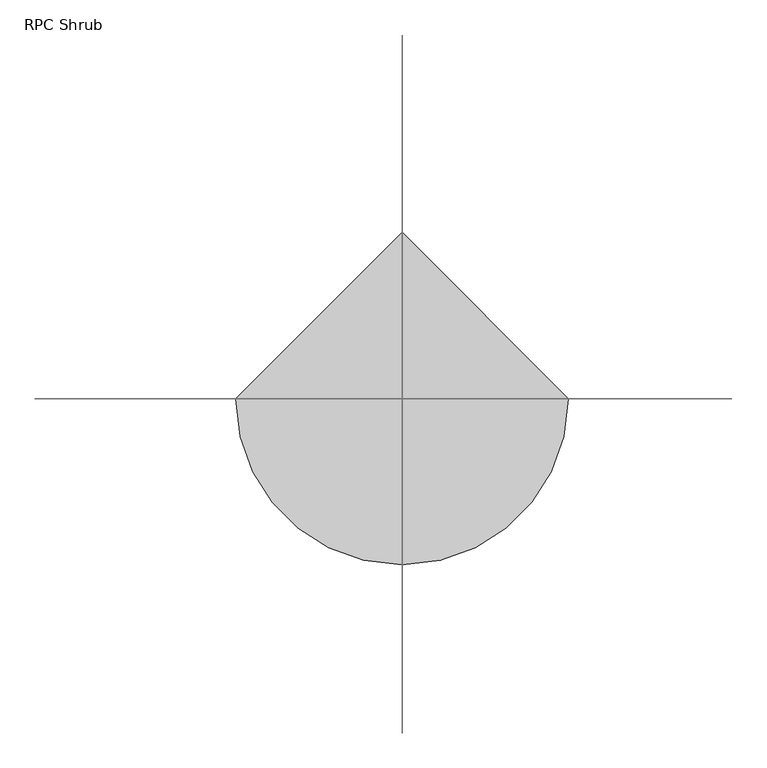
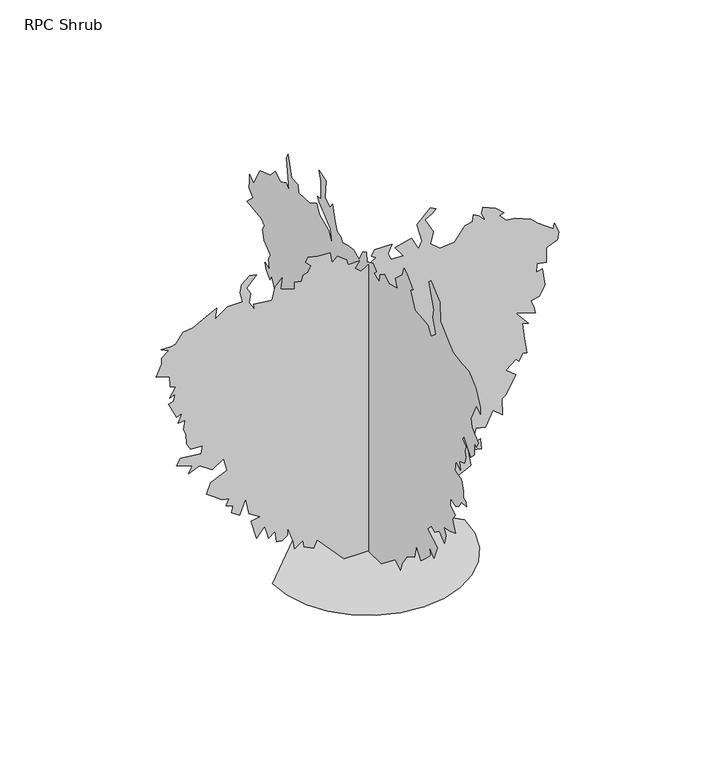
"""IFC4 building model written with IfcOpenShell, lengths in millimetres: geographic element geometry, RPC Shrub."""

from ifc_helpers import new_model, si_unit, origin, place, context, project, spatial, triangles, source, transform, mapped, element, save


def rpc_shrub_9ef344a8(model_context):
    return source(origin(), model_context, "Body", "Tessellation", [
        triangles([(-63.9369313, 2.6e-06, 2.5813025), (-98.6351404, 1.9e-06, 41.3616468), (-133.3335948, 1.1e-06, 80.1421467), (-143.538813, 2.7e-06, 59.7314513), (-168.0315495, 3.1e-06, 71.9778149), (-170.0726858, 2.1e-06, 90.347365), (-192.5245312, 3.9e-06, 76.0598514), (-194.5656857, 2.9e-06, 94.4296558), (-210.8940858, 9e-07, 139.3333375), (-210.8940858, 2.1e-06, 118.9223832), (-225.1818402, 3.4e-06, 108.7171649), (-239.469104, 3.9e-06, 110.7583103), (-243.5513948, 2.2e-06, 141.3742286), (-260.2917792, 3.7e-06, 128.4682213), (-264.2033864, 3e-06, 143.1357217), (-270.0860397, 2e-06, 163.8260649), (-290.4949502, 4.4e-06, 139.3333375), (-304.7824684, 2e-06, 190.3599468), (-282.331386, 8e-07, 194.4422376), (-310.9064223, 9e-07, 212.8117922), (-319.0699865, -1.4e-06, 257.7162279), (-335.3996584, 1.7e-06, 216.894083), (-355.8110942, 1.8e-06, 231.181583), (-351.7293303, 5e-07, 249.5511376), (-370.0986305, 9e-07, 255.674056), (-361.9325229, -4e-07, 272.003746), (-380.3043303, 2e-07, 276.0855281), (-401.9400736, 2e-07, 291.703997), (-421.1247311, 3e-07, 304.6605463), (-410.918995, -1.9e-06, 333.2355826), (-368.1987102, -4.9e-06, 351.9401459), (-376.2200229, -6.6e-06, 386.3038187), (-406.8371947, -4.1e-06, 367.9345184), (-439.493995, -4.1e-06, 390.385619), (-468.0690313, -2.1e-06, 378.137711), (-457.8632953, -3.5e-06, 394.4673829), (-498.6862032, -2.7e-06, 410.7970548), (-488.4805035, -4.1e-06, 427.1242195), (-435.4122311, -6.1e-06, 421.0002474), (-431.3304308, -7.5e-06, 441.4117195), (-461.9450955, -6.2e-06, 443.4538914), (-472.1508316, -6.9e-06, 461.8231553), (-474.1929671, -8.4e-06, 488.3560198), (-480.3169393, -9e-06, 502.6435561), (-476.2325955, -1.06e-05, 527.1367922), (-495.4832737, -9.7e-06, 526.35192), (-484.3987032, -1.16e-05, 549.5878564), (-498.6862032, -1.06e-05, 543.466464), (-519.0951319, -1.23e-05, 586.3290004), (-506.8497674, -1.3e-05, 590.4107643), (-502.7680035, -1.43e-05, 608.7800646), (-517.0555035, -1.33e-05, 602.6561288), (-500.7258316, -1.55e-05, 627.1493649), (-516.1995237, -1.52e-05, 634.2689884), (-517.0555035, -1.68e-05, 661.848337), (-551.7544756, -1.59e-05, 672.0540367), (-537.4644321, -1.84e-05, 702.6687378), (-538.1857907, -1.94e-05, 720.3319038), (-519.0951319, -2.1e-05, 733.2859097), (-539.506604, -2.07e-05, 743.4916094), (-512.7375257, -2.18e-05, 742.0895147), (-500.7258316, -2.25e-05, 745.5312378), (-482.3565313, -2.49e-05, 772.0666094), (-455.8236669, -2.62e-05, 774.1062378), (-423.1668666, -2.87e-05, 792.4755381), (-395.1176339, -3.08e-05, 806.3871162), (-398.6736305, -2.9e-05, 778.1880381), (-366.0168303, -3.17e-05, 800.6416821), (-327.2360942, -3.34e-05, 800.6416821), (-334.4166515, -3.47e-05, 827.9339842), (-330.1088113, -3.62e-05, 849.0616917), (-308.8667939, -3.81e-05, 865.9552826), (-290.4949502, -3.87e-05, 861.8734823), (-317.5358142, -3.58e-05, 834.0731443), (-306.8246221, -3.53e-05, 816.9688105), (-310.9064223, -3.36e-05, 792.4755381), (-296.6189042, -3.29e-05, 770.0245102), (-298.6610579, -3.37e-05, 784.3120102), (-251.0357672, -3.54e-05, 778.383593), (-243.5513948, -3.77e-05, 810.8473818), (-225.1818402, -3.97e-05, 831.2563105), (-228.2958943, -3.78e-05, 801.312208), (-192.5245312, -3.86e-05, 788.3937378), (-192.5245312, -3.97e-05, 806.7630381), (-173.5245645, -4.03e-05, 803.1613684), (-170.0726858, -4.14e-05, 819.0109823), (-157.8260678, -4.22e-05, 823.0927099), (-149.662004, -4.34e-05, 837.3802826), (-163.9495131, -4.36e-05, 851.6677826), (-157.8260678, -4.46e-05, 863.9131107), (-131.292195, -4.54e-05, 857.7916821), (-100.6760314, -4.66e-05, 855.7495102), (-94.5528496, -4.52e-05, 827.1745102), (-80.2653314, -4.65e-05, 839.4223818), (-56.9158573, -4.65e-05, 821.1673914), (-53.7314587, -4.57e-05, 806.7630381), (-23.1153655, -4.71e-05, 806.7630381), (-35.3616542, -4.56e-05, 790.4359097), (-19.0331746, -4.54e-05, 776.1484097), (19.7470164, -4.86e-05, 800.6416821), (7.5007532, -4.85e-05, 808.8052099), (15.1231208, -4.98e-05, 823.890263), (60.5683824, -5.17e-05, 823.0927099), (50.5958261, -4.99e-05, 799.816151), (58.5274868, -4.92e-05, 782.2723818), (91.1845505, -5.05e-05, 780.2302099), (68.732964, -5.13e-05, 810.8473818), (111.5952414, -5.38e-05, 821.0506107), (129.9650504, -5.25e-05, 786.3541821), (138.9452253, -5.4e-05, 804.6625122), (125.8830048, -5.64e-05, 853.7099545), (160.581223, -6e-05, 888.4063831), (174.868723, -6.01e-05, 880.2427826), (164.6635138, -5.91e-05, 870.0370829), (146.2937048, -5.76e-05, 859.8313105), (168.7455503, -5.62e-05, 819.0109823), (161.0930195, -5.4e-05, 788.6985884), (185.0742047, -5.39e-05, 767.9848818), (203.4434868, -5.48e-05, 770.0245102), (223.8544503, -5.58e-05, 772.0666094), (250.3885683, -5.9e-05, 806.7630381), (269.7101179, -6.01e-05, 811.2766434), (272.8393963, -6.13e-05, 829.2166821), (285.0872861, -6.15e-05, 823.0927099), (304.0839645, -6.12e-05, 803.1613684), (293.2508503, -6.21e-05, 827.1745102), (297.3326324, -6.31e-05, 841.4620102), (329.9894508, -6.37e-05, 827.1745102), (351.394031, -6.35e-05, 807.9441433), (340.0529354, -6.27e-05, 803.4457987), (358.5644508, -6.24e-05, 784.3120102), (381.0180948, -6.33e-05, 782.2723818), (422.1051581, -6.41e-05, 765.7470823), (440.2077596, -6.38e-05, 747.5734097), (481.0306675, -6.39e-05, 718.9984097), (483.0702959, -6.48e-05, 733.2859097), (495.3181675, -6.36e-05, 704.710837), (491.2364036, -6.23e-05, 684.2994375), (462.6588238, -6.03e-05, 672.0540367), (462.6588238, -5.8e-05, 633.273337), (438.1681312, -5.71e-05, 637.3550646), (436.1259593, -5.57e-05, 614.9040367), (452.4556312, -5.67e-05, 618.9857643), (458.5770598, -5.41e-05, 572.041464), (444.2895235, -5.19e-05, 545.5060925), (421.8384593, -5.07e-05, 541.4242922), (430.0020235, -4.98e-05, 521.0128201), (434.0863309, -4.91e-05, 504.6856916), (383.0577232, -4.78e-05, 521.0128201), (415.7145235, -4.69e-05, 482.2346274), (399.3873951, -4.64e-05, 486.3163914), (405.5087874, -4.42e-05, 443.4538914), (411.6327232, -4.2e-05, 402.6309471), (401.4269872, -4.17e-05, 404.673119), (391.2212874, -4.01e-05, 386.3038187), (383.0577232, -4.03e-05, 394.4673829), (356.5248588, -3.79e-05, 374.0559471), (383.0577232, -3.77e-05, 351.6048466), (356.5248588, -3.39e-05, 306.7001747), (346.3191227, -3.29e-05, 298.5365923), (348.3587511, -3.03e-05, 253.6334284), (323.4463909, -3.05e-05, 274.9933165), (303.4565864, -2.73e-05, 235.2636194), (278.9633503, -2.66e-05, 241.3868104), (266.8272088, -2.35e-05, 199.2829668), (291.2086966, -2.52e-05, 208.7297557), (293.2508503, -2.36e-05, 180.1547194), (258.5518782, -2.25e-05, 188.3190466), (266.7179858, -2.02e-05, 143.415374), (232.0187775, -1.77e-05, 127.0867195), (215.6903774, -1.54e-05, 100.5528377), (197.3205684, -1.5e-05, 106.6760195), (191.1973775, -1.2e-05, 61.7723423), (176.9098775, -1.3e-05, 88.306474), (150.3759956, -8.8e-06, 37.2796104), (132.0059414, -8.8e-06, 51.5671195), (68.732964, -3.2e-06, 2.5813025), (5e-07, 58.5086925, 0.0), (5.6e-06, 119.7410287, 55.1089), (6.1e-06, 137.5863239, 49.658565), (5.6e-06, 170.7679014, 104.0948725), (5.5e-06, 180.9731106, 91.8482545), (9.8e-06, 197.3017651, 73.4787044), (6.8e-06, 213.6304195, 87.7662181), (6.7e-06, 205.4660923, 93.8893999), (9.7e-06, 223.8356469, 144.9162635), (8.6e-06, 231.9999742, 112.2589454), (1e-05, 238.1231651, 136.7519272), (1.13e-05, 276.9033925, 128.5875999), (1.12e-05, 254.4523283, 148.9982999), (1.22e-05, 274.8637822, 151.0394453), (1.45e-05, 307.5205825, 171.4501453), (1.42e-05, 280.9851927, 191.8608363), (1.68e-05, 299.3544748, 232.6824725), (1.68e-05, 317.7263186, 214.3126635), (1.89e-05, 350.3043809, 228.0708535), (1.99e-05, 340.1773828, 261.2569819), (2.07e-05, 354.4649191, 265.338764), (2.22e-05, 356.5045112, 297.9955825), (2.36e-05, 393.2456552, 293.9138004), (2.61e-05, 411.6149554, 332.6945546), (2.58e-05, 397.3274554, 338.8184904), (2.92e-05, 438.1478199, 377.5992265), (2.82e-05, 405.4910196, 385.7627907), (2.9e-05, 411.6149554, 398.0081552), (2.55e-05, 417.7363478, 412.2956552), (2.48e-05, 395.2852836, 418.4196273), (2.73e-05, 415.6967194, 455.1581915), (2.98e-05, 436.1081915, 491.8993355), (2.95e-05, 444.2717557, 477.6118355), (3.11e-05, 460.5988841, 498.0207278), (3.2e-05, 466.7228199, 512.3082642), (3.07e-05, 446.3113841, 504.1447), (3.21e-05, 450.3956915, 530.6800715), (3.24e-05, 440.1899554, 547.0072), (3.47e-05, 470.8046202, 569.4583005), (3.61e-05, 476.928556, 595.9937084), (3.64e-05, 468.7649918, 610.2812084), (3.74e-05, 481.0103562, 622.5265366), (4.07e-05, 546.3265002, 630.6926805), (4.07e-05, 519.7910923, 657.2255087), (4.22e-05, 538.1603926, 673.5551805), (4.29e-05, 536.5677936, 692.1911797), (4.37e-05, 535.3943187, 712.0133709), (4.23e-05, 517.7489204, 698.0459095), (3.89e-05, 487.134292, 751.1141819), (3.76e-05, 440.1899554, 767.4438538), (3.77e-05, 419.7785196, 789.8948816), (3.6e-05, 395.2852836, 775.6073816), (3.55e-05, 370.7920475, 787.8553259), (3.44e-05, 358.546683, 775.6073816), (3.84e-05, 368.7524191, 857.250654), (3.88e-05, 362.6284833, 871.5382267), (3.56e-05, 346.2988114, 816.4303259), (3.43e-05, 317.7237751, 814.388154), (3.33e-05, 315.6841467, 793.9766819), (3.12e-05, 262.6158925, 798.0584822), (3.06e-05, 234.0411286, 814.388154), (2.9e-05, 219.7536105, 791.9370535), (2.65e-05, 180.9731106, 773.5677532), (2.43e-05, 162.603556, 740.9084095), (2.65e-05, 170.7679014, 783.7709822), (3.06e-05, 223.8356469, 824.5938538), (3.15e-05, 229.9590922, 836.8392546), (3.08e-05, 213.6301652, 838.8814264), (3.3e-05, 213.6301652, 887.8678986), (3.45e-05, 223.8356469, 912.3585548), (3.26e-05, 191.1785923, 902.1553986), (3.06e-05, 195.2606287, 853.1689264), (2.91e-05, 172.8087833, 840.9209822), (2.93e-05, 162.603556, 855.2085548), (2.71e-05, 150.356947, 816.4303259), (2.57e-05, 142.1926198, 793.9766819), (2.47e-05, 123.8230652, 787.8553259), (2.4e-05, 117.7001377, 777.6495535), (2.32e-05, 95.248047, 783.7709822), (2.23e-05, 68.7141651, 787.8553259), (2.06e-05, 43.1368564, 776.3617687), (2.13e-05, 25.8518877, 808.2641819), (2.09e-05, 9.5229755, 816.4303259), (1.98e-05, 7.4819061, 791.9370535), (1.91e-05, -19.0520211, 804.1824543), (1.78e-05, -35.3804508, 789.8948816), (1.78e-05, -25.1750781, 779.6891819), (1.63e-05, -49.6682165, 769.4834822), (1.72e-05, -51.7091075, 791.9370535), (1.69e-05, -72.1200574, 806.2245535), (1.54e-05, -92.5307528, 791.9370535), (1.42e-05, -129.2700982, 802.1428259), (1.56e-05, -121.105771, 824.5938538), (1.54e-05, -153.0015985, 852.691412), (1.61e-05, -159.8860075, 875.6199543), (1.52e-05, -172.1326437, 867.4564264), (1.28e-05, -200.7076618, 840.9209822), (1.3e-05, -188.4607894, 832.7574543), (1.02e-05, -208.8717347, 789.8948816), (8.5e-06, -245.6110801, 787.8553259), (7.4e-06, -268.0641973, 783.7709822), (5.8e-06, -280.3095436, 761.3198816), (5.7e-06, -303.1314609, 780.7331589), (8e-06, -290.5152796, 820.5121262), (8.8e-06, -294.5970617, 842.963154), (1.25e-05, -272.1459794, 906.2371988), (1.25e-05, -280.3095436, 914.4007267), (9.2e-06, -321.1299262, 879.7017546), (6.9e-06, -323.1720617, 828.675654), (4.3e-06, -354.6452497, 799.5291046), (2.2e-06, -380.3221344, 777.6495535), (1e-07, -421.1424989, 771.5255814), (-1.3e-06, -451.7596707, 769.4834822), (-3.9e-06, -482.3768789, 740.9084095), (-6.6e-06, -502.7857713, 700.0880814), (-7.4e-06, -502.7857713, 681.7187811), (-6e-06, -486.4586429, 696.0062811), (-2.7e-06, -459.9232349, 644.9801805), (-3.9e-06, -466.0472071, 624.5687084), (-6.3e-06, -494.6222071, 598.0333005), (-6.6e-06, -486.4586429, 581.7061721), (-5.9e-06, -476.2529068, 587.8301442), (-7.3e-06, -476.2529068, 555.1708005), (-7.3e-06, -459.9232349, 538.8436357), (-4.3e-06, -429.3086065, 577.6244081), (-4.5e-06, -423.1846707, 567.4186721), (-5.7e-06, -439.5143426, 555.1708005), (-6.2e-06, -433.3903705, 538.8436357), (-7.1e-06, -439.5143426, 524.5561357), (-7.6e-06, -431.3482349, 504.1447), (-7e-06, -408.8971344, 495.9810994), (-8.2e-06, -412.9789347, 473.5300352), (-6.6e-06, -392.5674625, 487.8175352), (-7.7e-06, -388.4856986, 459.2425352), (-9.4e-06, -419.1028705, 451.0764276), (-1.08e-05, -427.2664347, 426.5831915), (-1.17e-05, -428.2418112, 408.450105), (-1.23e-05, -437.4721707, 402.0924989), (-1.3e-05, -441.553971, 391.8867628), (-1.21e-05, -419.1028705, 389.844591), (-1.23e-05, -406.8549989, 371.4752907), (-1.22e-05, -394.6096344, 363.3117265), (-1.07e-05, -368.0767699, 369.4331188), (-7.3e-06, -368.0767699, 349.0242265), (-8.8e-06, -390.5278705, 336.7763186), (-9e-06, -378.2799625, 318.4070183), (-1.09e-05, -390.5278705, 287.7923899), (-1.03e-05, -366.0345981, 277.5866538), (-9.3e-06, -339.5017336, 273.5048717), (-1.05e-05, -347.6653341, 255.1330462), (-1.13e-05, -341.541362, 230.6413362), (-9.5e-06, -319.0902978, 249.0108726), (-9.2e-06, -298.6788438, 234.7233726), (-8.2e-06, -284.3913257, 242.8876998), (-8.2e-06, -266.0220254, 224.5181452), (-1.13e-05, -310.9241901, 200.0251635), (-1.22e-05, -294.5970617, 161.2446636), (-1.04e-05, -272.1459794, 181.6556089), (-1.16e-05, -278.2673899, 159.2037635), (-1.17e-05, -263.9798717, 142.8751181), (-1.15e-05, -235.4058709, 118.3821273), (-9.5e-06, -214.9951618, 144.9162635), (-1.06e-05, -205.8577653, 109.83274), (-1e-05, -174.1735256, 91.8482545), (-1.05e-05, -149.6807982, 57.1500454), (-6.7e-06, -143.5573621, 36.7393522), (-5.1e-06, -121.105771, 51.0268636), (-4.5e-06, -57.8322894, 2.0410923), (-249.8274834, 0.0, 0.0911396), (-243.2227266, -57.2440259, 0.0911358), (-224.4129918, -109.8131736, 0.091132), (-194.9037465, -156.2020027, 0.0911279), (-156.2020027, -194.9037465, 0.0911238), (-109.8131736, -224.4127374, 0.09112), (-57.2437715, -243.2227266, 0.0911167), (8.9e-06, -249.8274834, 0.0911137), (57.2440259, -243.2227266, 0.0911116), (109.8131736, -224.4127374, 0.0911454), (156.2020027, -194.9037465, 0.0911452), (194.9040008, -156.2020027, 0.0911459), (224.4127374, -109.8131736, 0.0911122), (243.2227266, -57.2437715, 0.0911147), (249.8274834, 2.18e-05, 0.0911177), (-3.49e-05, 249.8274834, 0.0911434)], [[59, 60, 61], [135, 136, 137], [51, 52, 53], [34, 35, 36], [149, 150, 151], [80, 81, 82], [172, 173, 174], [160, 161, 162], [96, 97, 98], [16, 17, 18], [16, 18, 19], [65, 66, 67], [147, 148, 149], [72, 73, 74], [71, 72, 74], [70, 71, 74], [45, 46, 47], [128, 129, 130], [6, 7, 8], [106, 107, 108], [106, 108, 109], [13, 14, 15], [102, 103, 104], [146, 147, 149], [152, 153, 154], [79, 80, 82], [166, 167, 168], [165, 166, 168], [122, 123, 124], [154, 155, 156], [112, 113, 114], [111, 112, 114], [111, 114, 115], [77, 78, 79], [21, 22, 23], [21, 23, 24], [83, 84, 85], [174, 175, 176], [36, 37, 38], [36, 38, 39], [34, 36, 39], [139, 140, 141], [55, 56, 57], [24, 25, 26], [126, 127, 128], [125, 126, 128], [125, 128, 130], [101, 102, 104], [100, 101, 104], [48, 49, 50], [47, 48, 50], [142, 143, 144], [3, 4, 5], [3, 5, 6], [110, 111, 115], [110, 115, 116], [110, 116, 117], [109, 110, 117], [69, 70, 74], [69, 74, 75], [69, 75, 76], [122, 124, 125], [157, 158, 159], [21, 24, 26], [93, 94, 95], [162, 163, 164], [170, 171, 172], [89, 90, 91], [88, 89, 91], [28, 29, 30], [28, 30, 31], [27, 28, 31], [26, 27, 31], [168, 169, 170], [11, 12, 13], [10, 11, 13], [9, 10, 13], [91, 92, 93], [88, 91, 93], [87, 88, 93], [13, 15, 16], [93, 95, 96], [21, 26, 31], [32, 33, 34], [32, 34, 39], [32, 39, 40], [79, 82, 83], [100, 104, 105], [53, 54, 55], [6, 8, 9], [64, 65, 67], [85, 86, 87], [57, 58, 59], [99, 100, 105], [55, 57, 59], [40, 41, 42], [40, 42, 43], [135, 137, 138], [135, 138, 139], [134, 135, 139], [142, 144, 145], [142, 145, 146], [152, 154, 156], [134, 139, 141], [157, 159, 160], [142, 146, 149], [62, 63, 64], [177, 1, 2], [176, 177, 2], [176, 2, 3], [85, 87, 93], [19, 20, 21], [125, 130, 131], [133, 134, 141], [132, 133, 141], [131, 132, 141], [174, 176, 3], [109, 117, 118], [85, 93, 96], [85, 96, 98], [83, 85, 98], [125, 131, 141], [125, 141, 142], [125, 142, 149], [122, 125, 149], [121, 122, 149], [120, 121, 149], [119, 120, 149], [118, 119, 149], [83, 98, 99], [47, 50, 51], [172, 174, 3], [59, 61, 62], [55, 59, 62], [55, 62, 64], [55, 64, 67], [53, 55, 67], [9, 13, 16], [9, 16, 19], [157, 160, 162], [168, 170, 172], [168, 172, 3], [165, 168, 3], [164, 165, 3], [164, 3, 6], [164, 6, 9], [164, 9, 19], [164, 19, 21], [164, 21, 31], [164, 31, 32], [162, 164, 32], [157, 162, 32], [157, 32, 40], [157, 40, 43], [157, 43, 44], [157, 44, 45], [157, 45, 47], [157, 47, 51], [157, 51, 53], [157, 53, 67], [157, 67, 68], [156, 157, 68], [152, 156, 68], [109, 118, 149], [106, 109, 149], [105, 106, 149], [99, 105, 149], [99, 149, 151], [99, 151, 152], [83, 99, 152], [79, 83, 152], [77, 79, 152], [77, 152, 68], [77, 68, 69], [76, 77, 69], [186, 187, 188], [188, 189, 190], [232, 233, 234], [231, 232, 234], [308, 309, 310], [211, 212, 213], [292, 293, 294], [246, 247, 248], [219, 220, 221], [246, 248, 249], [245, 246, 249], [250, 251, 252], [223, 224, 225], [202, 203, 204], [327, 328, 329], [259, 260, 261], [209, 210, 211], [209, 211, 213], [191, 192, 193], [243, 244, 245], [333, 334, 335], [332, 333, 335], [271, 272, 273], [315, 316, 317], [314, 315, 317], [342, 343, 344], [273, 274, 275], [258, 259, 261], [291, 292, 294], [271, 273, 275], [183, 184, 185], [182, 183, 185], [326, 327, 329], [205, 206, 207], [300, 301, 302], [299, 300, 302], [321, 322, 323], [297, 298, 299], [296, 297, 299], [262, 263, 264], [261, 262, 264], [296, 299, 302], [337, 338, 339], [200, 201, 202], [199, 200, 202], [323, 324, 325], [242, 243, 245], [242, 245, 249], [242, 249, 250], [242, 250, 252], [242, 252, 253], [237, 238, 239], [283, 284, 285], [282, 283, 285], [282, 285, 286], [281, 282, 286], [280, 281, 286], [280, 286, 287], [195, 196, 197], [194, 195, 197], [241, 242, 253], [241, 253, 254], [241, 254, 255], [234, 235, 236], [231, 234, 236], [227, 228, 229], [190, 191, 193], [179, 180, 181], [303, 304, 305], [229, 230, 231], [270, 271, 275], [269, 270, 275], [269, 275, 276], [197, 198, 199], [266, 267, 268], [265, 266, 268], [222, 223, 225], [221, 222, 225], [186, 188, 190], [182, 185, 186], [181, 182, 186], [204, 205, 207], [329, 330, 331], [323, 325, 326], [280, 287, 288], [321, 323, 326], [311, 312, 313], [335, 336, 337], [335, 337, 339], [332, 335, 339], [295, 296, 302], [277, 278, 279], [219, 221, 225], [219, 225, 226], [219, 226, 227], [219, 227, 229], [218, 219, 229], [218, 229, 231], [186, 190, 193], [306, 307, 308], [305, 306, 308], [303, 305, 308], [303, 308, 310], [311, 313, 314], [311, 314, 317], [311, 317, 318], [311, 318, 319], [311, 319, 320], [339, 340, 341], [258, 261, 264], [345, 178, 179], [344, 345, 179], [344, 179, 181], [216, 217, 218], [215, 216, 218], [215, 218, 231], [215, 231, 236], [215, 236, 237], [215, 237, 239], [215, 239, 240], [215, 240, 241], [341, 342, 344], [341, 344, 181], [339, 341, 181], [332, 339, 181], [332, 181, 186], [332, 186, 193], [332, 193, 194], [331, 332, 194], [279, 280, 288], [290, 291, 294], [289, 290, 294], [289, 294, 295], [288, 289, 295], [279, 288, 295], [279, 295, 302], [279, 302, 303], [279, 303, 310], [213, 214, 215], [209, 213, 215], [209, 215, 241], [208, 209, 241], [207, 208, 241], [326, 329, 331], [321, 326, 331], [321, 331, 194], [320, 321, 194], [311, 320, 194], [310, 311, 194], [279, 310, 194], [277, 279, 194], [276, 277, 194], [269, 276, 194], [268, 269, 194], [265, 268, 194], [264, 265, 194], [258, 264, 194], [258, 194, 197], [258, 197, 199], [258, 199, 202], [258, 202, 204], [258, 204, 207], [258, 207, 241], [258, 241, 255], [258, 255, 256], [257, 258, 256], [360, 361, 346], [359, 360, 346], [359, 346, 347], [358, 359, 347], [358, 347, 348], [358, 348, 349], [357, 358, 349], [356, 357, 349], [356, 349, 350], [356, 350, 351], [356, 351, 352], [356, 352, 353], [356, 353, 354], [356, 354, 355]], closed=False),
    ])


if __name__ == "__main__":
    model = new_model("IFC4")
    model_context = context("Model", 3, world=origin())
    ifc_project = project(units=[si_unit("LENGTHUNIT", "METRE", prefix="MILLI")], contexts=[model_context])
    site = spatial("IfcSite", under=ifc_project)
    building = spatial("IfcBuilding", under=site)
    placement = place(None, origin())
    rpc_shrub_shape = rpc_shrub_9ef344a8(model_context)
    element("IfcGeographicElement", 1, ObjectType="RPC Shrub", at=placement, inside=building, context=model_context, shape_type="MappedRepresentation", body=[
        mapped(rpc_shrub_shape, transform((0.0, 0.0, 0.0), x_axis=(1.0, 0.0, 0.0), y_axis=(0.0, 1.0, 0.0), z_axis=(0.0, 0.0, 1.0))),
    ])
    save(model, "model.ifc")

# Revit data of these elements
# Type "RPC Shrub"
#   built-in parameter 1005198 = "{2, 15},{39, RPC-16-G0FT-Q7G0-0DUH-W000-ST1L-LVER-AU},{1, 0},{1, 0},{2, 13},{1, 8},{5, Color},{1, 0},{1, 0},{3, 0.8},{3, 0.8},{3, 0.8},{1, 8},{7, BBoxMin},{1, 0},{1, 0},{1, 0},{1, 0},{1, 0},{1, 8},{7, BBoxMax},{1, 0},{1, 0},{1, 0},{1, 0},{1, 0},{2, 11},{9, RPCTypeId},{1, 0},{1, 0},{39, RPC-16-G0FT-Q7G0-0DUH-W000-ST1L-LVER-AU},{1, 6},{14, RPCPlantHeight},{1, 0},{1, 0},{1, 3},{2, 11},{7, keyword},{1, 0},{1, 0},{35, :RPCs:Shrubs [General]:Geometry:RPC},{2, 11},{8, category},{1, 0},{1, 0},{16, Shrubs [General]},{2, 11},{12, LocalizedUID},{1, 0},{1, 0},{10, Meadowlark},{2, 14},{6, Height},{1, 0},{1, 0},{1, 3},{1, 2},{16, Cast Reflections},{1, 0},{1, 0},{1, 0},{1, 2},{12, Cast Shadows},{1, 0},{1, 0},{1, 1},{1, 2},{9, Lock View},{1, 0},{1, 0},{1, 0},{1, 4},{5, ViewC},{1, 0},{1, 0},{1, 0},{21, assetlibrary_base.fbx},{1, 5},"
#   built-in parameter 1005195 = "RPC-16-G0FT-Q7G0-0DUH-W000-ST1L-LVER-AU"
#   Assembly Code = "G2050500"
#   Height = 3' - 0"
#   Default Elevation = 0
